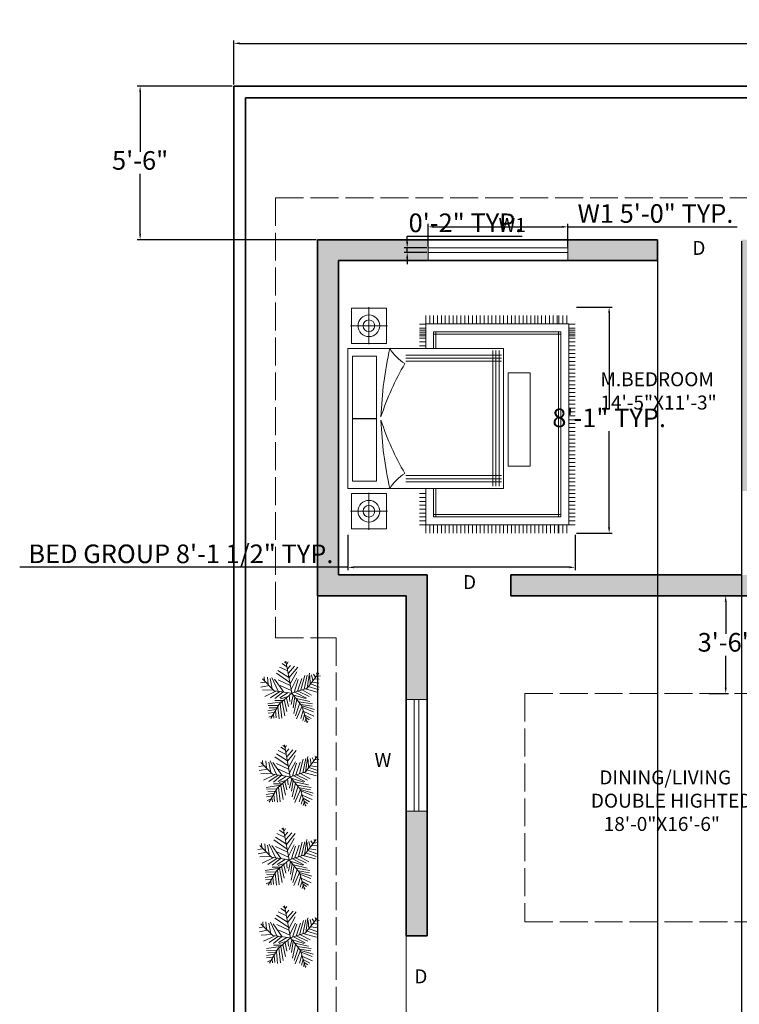
# Model space of a CAD drawing. Units: inches. Extents: x 1070 to 2371, y 645 to 1546.
# Tile 6 of 10: x 1070 to 1379, y 1014 to 1437. Entities that reach past the tile are written whole.
import ezdxf

# ---------------------------------------------------------------- set-up
doc = ezdxf.new("R2010")
doc.units = ezdxf.units.IN
doc.linetypes.add('ACAD_ISO02W100', pattern=[15, 12, -3])
for name, color, linetype, lineweight in [('A-ANNO-DIMS', 2, 'Continuous', 18), ('A-ANNO-TEXT', 7, 'Continuous', 18), ('A-AREA-IDEN', 7, 'Continuous', 18), ('A-DOOR', 4, 'Continuous', 18), ('A-FLOR-OVHD', 8, 'ACAD_ISO02W100', 13), ('A-FURN', 8, 'Continuous', 18), ('A-GLAZ', 4, 'Continuous', 18), ('A-ROOF-OVHD', 8, 'ACAD_ISO02W100', 13), ('A-WALL', 7, 'Continuous', 35), ('C-PROP', 7, 'Continuous', 35), ('L-PLNT-TREE', 94, 'Continuous', 13)]:
    doc.layers.add(name, color=color, linetype=linetype, lineweight=lineweight)
doc.layers.add('A-WALL-PATT', color=162, linetype='Continuous', lineweight=13, true_color=0x044ac3)
doc.styles.get("Standard").update_dxf_attribs({"font": 'arial.ttf'})
doc.dimstyles.new('ISO-25', dxfattribs={"dimtxt": 8, "dimasz": 2.5, "dimexe": 1.25, "dimexo": 0.625, "dimtad": 1, "dimtih": 1, "dimtoh": 1, "dimdec": 1, "dimlunit": 3, "dimtxsty": 'Standard', "dimcen": 2.5, "dimadec": 0, "dimazin": 0, "dimtfac": 1, "dimtdec": 1, "dimtmove": 0, "dimatfit": 3, "dimfxl": 1, "dimarcsym": 0})

# ---------------------------------------------------------------- blocks, each defined once
blk = doc.blocks.new('*U5')
for p, q in [((-8.737, 47.138), (-17.069, 52.711)), ((-10.186, 53.64), (-13.084, 55.962)), ((0, 0), (-10.5, 57)), ((-9.099, 51.782), (-6.563, 55.962)), ((-3.665, 19.273), (-27.574, 35.527)), ((-5.114, 28.097), (-24.676, 40.636)), ((-7.288, 39.707), (-21.778, 46.673)), ((-7.65, 43.423), (-2.578, 49.46)), ((-5.839, 35.992), (4.667, 48.067)), ((-5.114, 27.632), (10.463, 46.673)), ((-2.941, 16.486), (8.652, 37.85)), ((27, 9), (48, 36)), ((27.127, 9.056), (31.112, 35.992)), ((44.153, 36.456), (45.239, 32.741)), ((-47.498, 19.737), (-55.83, 18.344)), ((-31.5, 4.5), (-52.5, 25.5)), ((-48.585, 21.131), (-49.309, 29.026)), ((-43.513, 28.561), (-42.427, 15.558)), ((-38.442, 26.239), (-34.819, 7.663)), ((-35.544, 28.097), (-24.314, 3.947)), ((-14.533, 2.09), (-30.834, 25.31)), ((-24.314, 23.917), (-2.941, 13.7)), ((-1.129, 6.734), (9.014, 26.704)), ((3.942, 1.625), (11.187, 24.381)), ((10.101, 3.483), (17.708, 26.239)), ((16.259, 5.805), (23.142, 31.348)), ((22.055, 7.198), (27.489, 32.277)), ((31.836, 30.883), (32.561, 16.486)), ((35.096, 32.741), (37.27, 22.524)), ((36.183, 19.737), (48.137, 17.88)), ((38.719, 34.134), (41.979, 28.561)), ((40.53, 25.775), (48.862, 24.846)), ((43.791, 29.954), (51.036, 30.883)), ((-40.615, 13.7), (-55.105, 10.913)), ((-33.37, 6.269), (-52.207, 5.34)), ((-28.299, 3.483), (-47.86, -5.805)), ((-21.416, 3.018), (-38.079, -8.128)), ((0, 0), (-31.5, 4.5)), ((-15.982, 2.09), (-30.11, -9.521)), ((0, 0), (-22.5, -19.5)), ((-6.563, 1.161), (-21.416, -8.128)), ((-20.691, 13.7), (-1.129, 4.876)), ((0, 0), (27, 9)), ((0, 0), (18, -22.5)), ((6.478, 1.625), (26.04, -8.592)), ((11.187, 3.483), (30.749, -5.805)), ((18.07, 5.805), (35.096, -3.483)), ((24.229, 7.663), (46.688, 1.625)), ((29.662, 12.307), (48.137, 6.269)), ((33.285, 16.486), (48.862, 10.913)), ((-17.431, -15.094), (-42.789, -18.809)), ((-15.257, -12.772), (-30.11, -12.772)), ((-6.563, -5.805), (-19.967, -9.985)), ((-17.069, -15.094), (-12.721, -40.172)), ((-13.446, -11.378), (-8.737, -32.741)), ((-9.461, -8.592), (-6.201, -23.453)), ((-4.752, -3.483), (-3.665, -14.629)), ((2.493, -3.019), (-1.491, -20.202)), ((1.769, -2.555), (24.229, -9.521)), ((5.029, -6.27), (2.131, -25.775)), ((9.014, -11.378), (3.58, -35.992)), ((14.085, -16.951), (6.478, -40.172)), ((7.565, -9.056), (32.198, -14.629)), ((12.274, -15.094), (36.907, -18.809)), ((-28.299, -29.026), (-42.789, -31.348)), ((-24.314, -21.596), (-42.427, -22.06)), ((-30.834, -34.135), (-42.427, -35.528)), ((-26.849, -26.24), (-40.253, -25.775)), ((-22.5, -19.5), (-37.5, -45)), ((-29.023, -30.884), (-27.936, -43.887)), ((-25.038, -23.918), (-22.865, -45.281)), ((-20.691, -18.345), (-17.793, -44.352)), ((18.07, -22.524), (8.289, -45.745)), ((20.244, -30.419), (15.897, -44.816)), ((16.259, -19.738), (36.183, -22.989)), ((18, -22.5), (27, -52.5)), ((18.433, -22.524), (40.53, -29.026)), ((19.157, -25.311), (38.719, -33.206)), ((21.331, -32.741), (39.081, -40.636)), ((-34.457, -39.708), (-40.978, -42.494)), ((-32.646, -36.921), (-31.921, -44.352)), ((22.78, -37.85), (19.519, -48.532)), ((22.78, -38.314), (34.372, -44.816)), ((24.591, -45.745), (23.142, -50.854)), ((24.591, -43.423), (30.749, -47.603)), ((26.764, -49.925), (28.213, -50.854))]:
    blk.add_line(p, q)
blk = doc.blocks.new('A$C462B680F')
for p, q in [((2.33, 2.918, -0.291), (0.53, 2.918, -0.291)), ((0.53, 2.918, -0.291), (0.53, 0.918, -0.291)), ((2.33, 0.918, -0.291), (2.33, 2.918, -0.291)), ((0.011, 2.874, -0.291), (0.465, 2.874, -0.291)), ((0.011, 2.424, -0.291), (0.011, 2.874, -0.291)), ((0.238, 2.649, -0.561), (0.238, 2.887, -0.561)), ((0.465, 2.874, -0.291), (0.465, 2.424, -0.291)), ((1.434, 2.861, -0.291), (0.627, 2.861, -0.291)), ((0.627, 2.861, -0.291), (0.627, 2.55, -0.291)), ((1.43, 2.861, -0.291), (1.43, 2.55, -0.291)), ((2.237, 2.861, -0.291), (1.43, 2.861, -0.291)), ((1.434, 2.55, -0.291), (1.434, 2.861, -0.291)), ((2.237, 2.55, -0.291), (2.237, 2.861, -0.291)), ((2.849, 2.874, -0.291), (2.395, 2.874, -0.291)), ((2.395, 2.874, -0.291), (2.395, 2.424, -0.291)), ((2.622, 2.649, -0.561), (2.622, 2.887, -0.561)), ((2.849, 2.424, -0.291), (2.849, 2.874, -0.291)), ((0.238, 2.649, -0.561), (0, 2.649, -0.561)), ((0.238, 2.649, -0.561), (0.238, 2.411, -0.561)), ((0.238, 2.649, -0.561), (0.476, 2.649, -0.561)), ((0.627, 2.55, -0.291), (1.434, 2.55, -0.291)), ((1.43, 2.55, -0.291), (2.237, 2.55, -0.291)), ((2.622, 2.649, -0.561), (2.384, 2.649, -0.561)), ((2.622, 2.649, -0.561), (2.622, 2.411, -0.561)), ((2.622, 2.649, -0.561), (2.861, 2.649, -0.561)), ((0.465, 2.424, -0.291), (0.011, 2.424, -0.291)), ((2.395, 2.424, -0.291), (2.849, 2.424, -0.291)), ((0.615, 2.176, -0.291), (0.615, 0.947, -0.291)), ((0.655, 2.176, -0.291), (0.655, 0.947, -0.291)), ((0.695, 2.176, -0.291), (0.695, 0.947, -0.291)), ((2.165, 2.176, -0.291), (2.165, 0.947, -0.291)), ((2.205, 2.176, -0.291), (2.205, 0.947, -0.291)), ((2.245, 2.176, -0.291), (2.245, 0.947, -0.291)), ((0.215, 1.918, -0.291), (0.105, 1.918, -0.291)), ((0.215, 1.918, -0.291), (0.215, 0.082, -0.291)), ((0.53, 1.918, -0.291), (0.215, 1.918, -0.291)), ((0.219, 1.918, -0.291), (0.219, 2, -0.291)), ((0.269, 1.918, -0.291), (0.269, 2, -0.291)), ((0.296, 1.918, -0.291), (0.296, 2, -0.291)), ((0.319, 1.918, -0.291), (0.319, 2, -0.291)), ((0.346, 1.918, -0.291), (0.346, 2, -0.291)), ((0.369, 1.918, -0.291), (0.369, 2, -0.291)), ((0.396, 1.918, -0.291), (0.396, 2, -0.291)), ((0.446, 1.918, -0.291), (0.446, 2, -0.291)), ((0.496, 1.918, -0.291), (0.496, 2, -0.291)), ((2.33, 1.918, -0.291), (2.796, 1.918, -0.291)), ((2.396, 1.918, -0.291), (2.396, 2, -0.291)), ((2.446, 1.918, -0.291), (2.446, 2, -0.291)), ((2.496, 1.918, -0.291), (2.496, 2, -0.291)), ((2.546, 1.918, -0.291), (2.546, 2, -0.291)), ((2.596, 1.918, -0.291), (2.596, 2, -0.291)), ((2.646, 1.918, -0.291), (2.646, 2, -0.291)), ((2.696, 1.918, -0.291), (2.696, 2, -0.291)), ((2.746, 1.918, -0.291), (2.746, 2, -0.291)), ((2.796, 1.918, -0.291), (2.796, 2, -0.291)), ((2.796, 1.918, -0.291), (2.796, 0.082, -0.291)), ((2.796, 1.918, -0.291), (2.906, 1.918, -0.291)), ((0.215, 1.868, -0.291), (0.105, 1.868, -0.291)), ((0.215, 1.818, -0.291), (0.105, 1.818, -0.291)), ((0.315, 1.818, -0.291), (0.315, 0.182, -0.291)), ((0.53, 1.818, -0.291), (0.315, 1.818, -0.291)), ((0.53, 1.788, -0.291), (0.315, 1.788, -0.291)), ((0.345, 1.818, -0.291), (0.345, 0.182, -0.291)), ((2.33, 1.818, -0.291), (2.696, 1.818, -0.291)), ((2.33, 1.788, -0.291), (2.696, 1.788, -0.291)), ((2.666, 1.818, -0.291), (2.666, 0.182, -0.291)), ((2.696, 1.818, -0.291), (2.696, 0.182, -0.291)), ((2.796, 1.868, -0.291), (2.906, 1.868, -0.291)), ((2.796, 1.818, -0.291), (2.906, 1.818, -0.291)), ((0.215, 1.768, -0.291), (0.105, 1.768, -0.291)), ((0.215, 1.718, -0.291), (0.105, 1.718, -0.291)), ((0.215, 1.668, -0.291), (0.105, 1.668, -0.291)), ((2.796, 1.768, -0.291), (2.906, 1.768, -0.291)), ((2.796, 1.718, -0.291), (2.906, 1.718, -0.291)), ((2.796, 1.668, -0.291), (2.906, 1.668, -0.291)), ((0.215, 1.618, -0.291), (0.105, 1.618, -0.291)), ((0.215, 1.568, -0.291), (0.105, 1.568, -0.291)), ((2.796, 1.618, -0.291), (2.906, 1.618, -0.291)), ((2.796, 1.568, -0.291), (2.906, 1.568, -0.291)), ((0.215, 1.518, -0.291), (0.105, 1.518, -0.291)), ((0.215, 1.468, -0.291), (0.105, 1.468, -0.291)), ((0.215, 1.418, -0.291), (0.105, 1.418, -0.291)), ((2.796, 1.518, -0.291), (2.906, 1.518, -0.291)), ((2.796, 1.468, -0.291), (2.906, 1.468, -0.291)), ((2.796, 1.418, -0.291), (2.906, 1.418, -0.291)), ((0.215, 1.368, -0.291), (0.105, 1.368, -0.291)), ((0.215, 1.318, -0.291), (0.105, 1.318, -0.291)), ((0.215, 1.268, -0.291), (0.105, 1.268, -0.291)), ((2.796, 1.368, -0.291), (2.906, 1.368, -0.291)), ((2.796, 1.318, -0.291), (2.906, 1.318, -0.291)), ((2.796, 1.268, -0.291), (2.906, 1.268, -0.291)), ((0.215, 1.218, -0.291), (0.105, 1.218, -0.291)), ((0.215, 1.168, -0.291), (0.105, 1.168, -0.291)), ((2.796, 1.218, -0.291), (2.906, 1.218, -0.291)), ((2.796, 1.168, -0.291), (2.906, 1.168, -0.291)), ((0.215, 1.118, -0.291), (0.105, 1.118, -0.291)), ((0.215, 1.068, -0.291), (0.105, 1.068, -0.291)), ((0.215, 1.018, -0.291), (0.105, 1.018, -0.291)), ((0.558, 1.057, -0.291), (2.299, 1.057, -0.291)), ((0.558, 1.017, -0.291), (2.299, 1.017, -0.291)), ((2.796, 1.118, -0.291), (2.906, 1.118, -0.291)), ((2.796, 1.068, -0.291), (2.906, 1.068, -0.291)), ((2.796, 1.018, -0.291), (2.906, 1.018, -0.291)), ((0.215, 0.968, -0.291), (0.105, 0.968, -0.291)), ((0.215, 0.918, -0.291), (0.105, 0.918, -0.291)), ((0.53, 0.918, -0.291), (2.33, 0.918, -0.291)), ((0.558, 0.977, -0.291), (2.299, 0.977, -0.291)), ((2.796, 0.968, -0.291), (2.906, 0.968, -0.291)), ((2.796, 0.918, -0.291), (2.906, 0.918, -0.291)), ((0.215, 0.868, -0.291), (0.105, 0.868, -0.291)), ((0.215, 0.818, -0.291), (0.105, 0.818, -0.291)), ((0.215, 0.768, -0.291), (0.105, 0.768, -0.291)), ((0.844, 0.859, -0.291), (0.844, 0.579, -0.291)), ((2.044, 0.859, -0.291), (0.844, 0.859, -0.291)), ((2.044, 0.579, -0.291), (2.044, 0.859, -0.291)), ((2.796, 0.868, -0.291), (2.906, 0.868, -0.291)), ((2.796, 0.818, -0.291), (2.906, 0.818, -0.291)), ((2.796, 0.768, -0.291), (2.906, 0.768, -0.291)), ((0.215, 0.718, -0.291), (0.105, 0.718, -0.291)), ((0.215, 0.668, -0.291), (0.105, 0.668, -0.291)), ((2.796, 0.718, -0.291), (2.906, 0.718, -0.291)), ((2.796, 0.668, -0.291), (2.906, 0.668, -0.291)), ((0.215, 0.618, -0.291), (0.105, 0.618, -0.291)), ((0.215, 0.568, -0.291), (0.105, 0.568, -0.291)), ((0.215, 0.518, -0.291), (0.105, 0.518, -0.291)), ((0.844, 0.579, -0.291), (2.044, 0.579, -0.291)), ((2.796, 0.618, -0.291), (2.906, 0.618, -0.291)), ((2.796, 0.568, -0.291), (2.906, 0.568, -0.291)), ((2.796, 0.518, -0.291), (2.906, 0.518, -0.291)), ((2.796, 0.516, -0.291), (2.906, 0.516, -0.291)), ((0.215, 0.48, -0.291), (0.105, 0.48, -0.291)), ((0.215, 0.43, -0.291), (0.105, 0.43, -0.291)), ((0.215, 0.38, -0.291), (0.105, 0.38, -0.291)), ((2.796, 0.466, -0.291), (2.906, 0.466, -0.291)), ((2.796, 0.416, -0.291), (2.906, 0.416, -0.291)), ((0.215, 0.33, -0.291), (0.105, 0.33, -0.291)), ((0.215, 0.28, -0.291), (0.105, 0.28, -0.291)), ((2.796, 0.366, -0.291), (2.906, 0.366, -0.291)), ((2.796, 0.316, -0.291), (2.906, 0.316, -0.291)), ((2.796, 0.266, -0.291), (2.906, 0.266, -0.291)), ((0.215, 0.23, -0.291), (0.105, 0.23, -0.291)), ((0.215, 0.207, -0.291), (0.105, 0.207, -0.291)), ((0.215, 0.207, -0.291), (0.105, 0.207, -0.291)), ((0.215, 0.157, -0.291), (0.105, 0.157, -0.291)), ((2.696, 0.212, -0.291), (0.315, 0.212, -0.291)), ((2.696, 0.182, -0.291), (0.315, 0.182, -0.291)), ((2.796, 0.216, -0.291), (2.906, 0.216, -0.291)), ((2.796, 0.207, -0.291), (2.906, 0.207, -0.291)), ((2.796, 0.207, -0.291), (2.906, 0.207, -0.291)), ((2.796, 0.157, -0.291), (2.906, 0.157, -0.291)), ((0.215, 0.107, -0.291), (0.105, 0.107, -0.291)), ((2.796, 0.082, -0.291), (0.215, 0.082, -0.291)), ((0.219, 0.082, -0.291), (0.219, 0, -0.291)), ((0.269, 0.082, -0.291), (0.269, 0, -0.291)), ((0.296, 0.082, -0.291), (0.296, 0, -0.291)), ((0.319, 0.082, -0.291), (0.319, 0, -0.291)), ((0.346, 0.082, -0.291), (0.346, 0, -0.291)), ((0.369, 0.082, -0.291), (0.369, 0, -0.291)), ((0.396, 0.082, -0.291), (0.396, 0, -0.291)), ((0.446, 0.082, -0.291), (0.446, 0, -0.291)), ((0.496, 0.082, -0.291), (0.496, 0, -0.291)), ((0.546, 0.082, -0.291), (0.546, 0, -0.291)), ((0.596, 0.082, -0.291), (0.596, 0, -0.291)), ((0.646, 0.082, -0.291), (0.646, 0, -0.291)), ((0.696, 0.082, -0.291), (0.696, 0, -0.291)), ((0.746, 0.082, -0.291), (0.746, 0, -0.291)), ((0.796, 0.082, -0.291), (0.796, 0, -0.291)), ((0.846, 0.082, -0.291), (0.846, 0, -0.291)), ((0.896, 0.082, -0.291), (0.896, 0, -0.291)), ((0.946, 0.082, -0.291), (0.946, 0, -0.291)), ((0.996, 0.082, -0.291), (0.996, 0, -0.291)), ((1.046, 0.082, -0.291), (1.046, 0, -0.291)), ((1.096, 0.082, -0.291), (1.096, 0, -0.291)), ((1.146, 0.082, -0.291), (1.146, 0, -0.291)), ((1.196, 0.082, -0.291), (1.196, 0, -0.291)), ((1.246, 0.082, -0.291), (1.246, 0, -0.291)), ((1.296, 0.082, -0.291), (1.296, 0, -0.291)), ((1.346, 0.082, -0.291), (1.346, 0, -0.291)), ((1.346, 0.082, -0.291), (1.346, 0, -0.291)), ((1.396, 0.082, -0.291), (1.396, 0, -0.291)), ((1.396, 0.082, -0.291), (1.396, 0, -0.291)), ((1.446, 0.082, -0.291), (1.446, 0, -0.291)), ((1.446, 0.082, -0.291), (1.446, 0, -0.291)), ((1.496, 0.082, -0.291), (1.496, 0, -0.291)), ((1.496, 0.082, -0.291), (1.496, 0, -0.291)), ((1.546, 0.082, -0.291), (1.546, 0, -0.291)), ((1.596, 0.082, -0.291), (1.596, 0, -0.291)), ((1.646, 0.082, -0.291), (1.646, 0, -0.291)), ((1.696, 0.082, -0.291), (1.696, 0, -0.291)), ((1.746, 0.082, -0.291), (1.746, 0, -0.291)), ((1.796, 0.082, -0.291), (1.796, 0, -0.291)), ((1.846, 0.082, -0.291), (1.846, 0, -0.291)), ((1.846, 0.082, -0.291), (1.846, 0, -0.291)), ((1.896, 0.082, -0.291), (1.896, 0, -0.291)), ((1.946, 0.082, -0.291), (1.946, 0, -0.291)), ((1.996, 0.082, -0.291), (1.996, 0, -0.291)), ((2.046, 0.082, -0.291), (2.046, 0, -0.291)), ((2.096, 0.082, -0.291), (2.096, 0, -0.291)), ((2.146, 0.082, -0.291), (2.146, 0, -0.291)), ((2.196, 0.082, -0.291), (2.196, 0, -0.291)), ((2.246, 0.082, -0.291), (2.246, 0, -0.291)), ((2.296, 0.082, -0.291), (2.296, 0, -0.291)), ((2.346, 0.082, -0.291), (2.346, 0, -0.291)), ((2.396, 0.082, -0.291), (2.396, 0, -0.291)), ((2.446, 0.082, -0.291), (2.446, 0, -0.291)), ((2.496, 0.082, -0.291), (2.496, 0, -0.291)), ((2.546, 0.082, -0.291), (2.546, 0, -0.291)), ((2.596, 0.082, -0.291), (2.596, 0, -0.291)), ((2.646, 0.082, -0.291), (2.646, 0, -0.291)), ((2.696, 0.082, -0.291), (2.696, 0, -0.291)), ((2.746, 0.082, -0.291), (2.746, 0, -0.291)), ((2.796, 0.107, -0.291), (2.906, 0.107, -0.291)), ((2.796, 0.082, -0.291), (2.796, 0, -0.291))]:
    blk.add_line(p, q)
for centre, radius in [((0.238, 2.649, -0.561), 0.139), ((2.622, 2.649, -0.561), 0.139), ((0.238, 2.649, -0.561), 0.075), ((2.622, 2.649, -0.561), 0.075)]:
    blk.add_circle(centre, radius)
for centre, radius, start, end in [((1.618, -2.572, -0.291), 5.071, 92.3872, 102.3913), ((2.601, -1.074, -0.291), 3.763, 108.5127, 119.9306), ((1.243, -2.572, -0.291), 5.071, 77.6087, 87.6128), ((0.259, -1.074, -0.291), 3.763, 60.0694, 71.4873), ((0.231, 1.886, -0.291), 0.578, 31.4118, 58.8491), ((2.63, 1.886, -0.291), 0.578, 121.1509, 148.5882)]:
    blk.add_arc(centre, radius, start, end)
blk = doc.blocks.new('*D11')
at = {"layer": 'A-ANNO-DIMS', "color": 0, "lineweight": -2, "transparency": 16777216}
for p, q in [((1162.11, 1409.4), (1162.11, 1428.36)), ((1164.61, 1427.11), (1639.61, 1427.11)), ((1642.11, 1409.4), (1642.11, 1428.36))]:
    blk.add_line(p, q, dxfattribs=at)
at = {"layer": 'A-ANNO-DIMS', "color": 0, "transparency": 16777216}
for points in [[(1164.61, 1427.53), (1164.61, 1426.7), (1162.11, 1427.11)], [(1639.61, 1427.53), (1639.61, 1426.7), (1642.11, 1427.11)]]:
    blk.add_solid(points, dxfattribs=at)
at = {"layer": 'Defpoints', "color": 0, "transparency": 16777216}
for p in [(1642.11, 1427.11), (1162.11, 1408.77), (1642.11, 1408.77)]:
    blk.add_point(p, dxfattribs=at)
at = {"layer": 'A-ANNO-DIMS', "color": 0, "transparency": 16777216, "insert": (1402.11, 1431.82), "char_height": 8, "attachment_point": 5}
blk.add_mtext("40'", dxfattribs=at)
blk = doc.blocks.new('*D13')
at = {"layer": 'A-ANNO-DIMS', "color": 0, "lineweight": -2, "transparency": 16777216}
for p, q in [((1366.14, 1189.77), (1374.63, 1189.77)), ((1373.38, 1187.27), (1373.38, 1173.48)), ((1373.38, 1150.27), (1373.38, 1164.06)), ((1366.14, 1147.77), (1374.63, 1147.77))]:
    blk.add_line(p, q, dxfattribs=at)
at = {"layer": 'A-ANNO-DIMS', "color": 0, "transparency": 16777216}
for points in [[(1372.97, 1187.27), (1373.8, 1187.27), (1373.38, 1189.77)], [(1372.97, 1150.27), (1373.8, 1150.27), (1373.38, 1147.77)]]:
    blk.add_solid(points, dxfattribs=at)
at = {"layer": 'Defpoints', "color": 0, "transparency": 16777216}
for p in [(1365.51, 1189.77), (1365.51, 1147.77), (1373.38, 1147.77)]:
    blk.add_point(p, dxfattribs=at)
at = {"layer": 'A-ANNO-DIMS', "color": 0, "transparency": 16777216, "insert": (1373.38, 1168.77), "char_height": 8, "attachment_point": 5}
blk.add_mtext('3\'-6"', dxfattribs=at)
blk = doc.blocks.new('GLAZ-48IN')
for p, q in [((0, 48), (0, 0)), ((2, 48), (2, 0))]:
    blk.add_line(p, q)
blk = doc.blocks.new('GLAZ-60IN')
for p, q in [((60, 2), (0, 2)), ((60, 0), (0, 0))]:
    blk.add_line(p, q)
blk = doc.blocks.new('*D27')
at = {"layer": 'A-ANNO-DIMS', "color": 0, "lineweight": -2, "transparency": 16777216}
for p, q in [((1211.17, 1216.02), (1211.17, 1200.77)), ((1308.69, 1216.02), (1308.69, 1200.77)), ((1211.17, 1202.02), (1070.2, 1202.02)), ((1306.19, 1202.02), (1213.67, 1202.02))]:
    blk.add_line(p, q, dxfattribs=at)
at = {"layer": 'A-ANNO-DIMS', "color": 0, "transparency": 16777216}
for points in [[(1213.67, 1202.44), (1213.67, 1201.6), (1211.17, 1202.02)], [(1306.19, 1202.44), (1306.19, 1201.6), (1308.69, 1202.02)]]:
    blk.add_solid(points, dxfattribs=at)
at = {"layer": 'Defpoints', "color": 0, "transparency": 16777216}
for p in [(1211.17, 1216.65), (1308.69, 1216.65), (1211.17, 1202.02)]:
    blk.add_point(p, dxfattribs=at)
at = {"layer": 'A-ANNO-DIMS', "color": 0, "transparency": 16777216, "insert": (1139.43, 1206.78), "char_height": 8, "attachment_point": 5}
blk.add_mtext('BED GROUP 8\'-1 1/2" TYP.', dxfattribs=at)
blk = doc.blocks.new('*D28')
at = {"layer": 'A-ANNO-DIMS', "color": 0, "lineweight": -2, "transparency": 16777216}
for p, q in [((1309.32, 1313.75), (1324.57, 1313.75)), ((1323.32, 1311.25), (1323.32, 1269.91)), ((1323.32, 1219.15), (1323.32, 1260.49)), ((1309.32, 1216.65), (1324.57, 1216.65))]:
    blk.add_line(p, q, dxfattribs=at)
at = {"layer": 'A-ANNO-DIMS', "color": 0, "transparency": 16777216}
for points in [[(1322.9, 1311.25), (1323.74, 1311.25), (1323.32, 1313.75)], [(1322.9, 1219.15), (1323.74, 1219.15), (1323.32, 1216.65)]]:
    blk.add_solid(points, dxfattribs=at)
at = {"layer": 'Defpoints', "color": 0, "transparency": 16777216}
for p in [(1308.69, 1313.75), (1308.69, 1216.65), (1323.32, 1216.65)]:
    blk.add_point(p, dxfattribs=at)
at = {"layer": 'A-ANNO-DIMS', "color": 0, "transparency": 16777216, "insert": (1323.32, 1265.2), "char_height": 8, "attachment_point": 5}
blk.add_mtext('8\'-1" TYP.', dxfattribs=at)
blk = doc.blocks.new('*D41')
at = {"layer": 'A-ANNO-DIMS', "color": 0, "lineweight": -2, "transparency": 16777216}
for p, q in [((1245.61, 1339.9), (1245.61, 1349.52)), ((1305.61, 1339.9), (1305.61, 1349.52)), ((1248.11, 1348.27), (1303.11, 1348.27)), ((1305.61, 1348.27), (1378.32, 1348.27))]:
    blk.add_line(p, q, dxfattribs=at)
at = {"layer": 'A-ANNO-DIMS', "color": 0, "transparency": 16777216}
for points in [[(1248.11, 1348.69), (1248.11, 1347.86), (1245.61, 1348.27)], [(1303.11, 1348.69), (1303.11, 1347.86), (1305.61, 1348.27)]]:
    blk.add_solid(points, dxfattribs=at)
at = {"layer": 'Defpoints', "color": 0, "transparency": 16777216}
for p in [(1305.61, 1348.27), (1245.61, 1339.27), (1305.61, 1339.27)]:
    blk.add_point(p, dxfattribs=at)
at = {"layer": 'A-ANNO-DIMS', "color": 0, "transparency": 16777216, "insert": (1343.22, 1352.98), "char_height": 8, "attachment_point": 5}
blk.add_mtext('W1 5\'-0" TYP.', dxfattribs=at)
blk = doc.blocks.new('*D42')
at = {"layer": 'A-ANNO-DIMS', "color": 0, "lineweight": -2, "transparency": 16777216}
for p, q in [((1236.61, 1341.77), (1236.61, 1344.27)), ((1236.61, 1344.27), (1286, 1344.27)), ((1244.99, 1339.27), (1235.36, 1339.27)), ((1244.99, 1337.27), (1235.36, 1337.27)), ((1236.61, 1337.27), (1236.61, 1339.27)), ((1236.61, 1334.77), (1236.61, 1332.27))]:
    blk.add_line(p, q, dxfattribs=at)
at = {"layer": 'A-ANNO-DIMS', "color": 0, "transparency": 16777216}
for points in [[(1236.2, 1341.77), (1237.03, 1341.77), (1236.61, 1339.27)], [(1236.2, 1334.77), (1237.03, 1334.77), (1236.61, 1337.27)]]:
    blk.add_solid(points, dxfattribs=at)
at = {"layer": 'Defpoints', "color": 0, "transparency": 16777216}
for p in [(1236.61, 1339.27), (1245.61, 1339.27), (1245.61, 1337.27)]:
    blk.add_point(p, dxfattribs=at)
at = {"layer": 'A-ANNO-DIMS', "color": 0, "transparency": 16777216, "insert": (1261.62, 1348.98), "char_height": 8, "attachment_point": 5}
blk.add_mtext('0\'-2" TYP.', dxfattribs=at)
blk = doc.blocks.new('*D47')
at = {"layer": 'A-ANNO-DIMS', "color": 0, "lineweight": -2, "transparency": 16777216}
for p, q in [((1162.11, 1408.15), (1162.11, 647.32)), ((1198.11, 1342.15), (1198.11, 647.32)), ((1164.61, 648.57), (1195.61, 648.57))]:
    blk.add_line(p, q, dxfattribs=at)
at = {"layer": 'A-ANNO-DIMS', "color": 0, "transparency": 16777216}
for points in [[(1164.61, 648.99), (1164.61, 648.16), (1162.11, 648.57)], [(1195.61, 648.99), (1195.61, 648.16), (1198.11, 648.57)]]:
    blk.add_solid(points, dxfattribs=at)
at = {"layer": 'Defpoints', "color": 0, "transparency": 16777216}
for p in [(1162.11, 1408.77), (1198.11, 1342.77), (1198.11, 648.57)]:
    blk.add_point(p, dxfattribs=at)
at = {"layer": 'A-ANNO-DIMS', "color": 0, "transparency": 16777216, "insert": (1180.11, 653.28), "char_height": 8, "attachment_point": 5}
blk.add_mtext('3\'-0"', dxfattribs=at)
blk = doc.blocks.new('*D48')
at = {"layer": 'A-ANNO-DIMS', "color": 0, "lineweight": -2, "transparency": 16777216}
for p, q in [((1161.49, 1408.77), (1120.66, 1408.77)), ((1121.91, 1406.27), (1121.91, 1380.48)), ((1121.91, 1345.27), (1121.91, 1371.06)), ((1197.49, 1342.77), (1120.66, 1342.77))]:
    blk.add_line(p, q, dxfattribs=at)
at = {"layer": 'A-ANNO-DIMS', "color": 0, "transparency": 16777216}
for points in [[(1121.5, 1406.27), (1122.33, 1406.27), (1121.91, 1408.77)], [(1121.5, 1345.27), (1122.33, 1345.27), (1121.91, 1342.77)]]:
    blk.add_solid(points, dxfattribs=at)
at = {"layer": 'Defpoints', "color": 0, "transparency": 16777216}
for p in [(1162.11, 1408.77), (1121.91, 1342.77), (1198.11, 1342.77)]:
    blk.add_point(p, dxfattribs=at)
at = {"layer": 'A-ANNO-DIMS', "color": 0, "transparency": 16777216, "insert": (1121.91, 1375.77), "char_height": 8, "attachment_point": 5}
blk.add_mtext('5\'-6"', dxfattribs=at)
blk = doc.blocks.new('*D49')
at = {"layer": 'A-ANNO-DIMS', "color": 0, "lineweight": -2, "transparency": 16777216}
for p, q in [((1344.11, 1342.15), (1344.11, 647.32)), ((1380.11, 1342.15), (1380.11, 647.32)), ((1346.61, 648.57), (1377.61, 648.57))]:
    blk.add_line(p, q, dxfattribs=at)
at = {"layer": 'A-ANNO-DIMS', "color": 0, "transparency": 16777216}
for points in [[(1346.61, 648.99), (1346.61, 648.16), (1344.11, 648.57)], [(1377.61, 648.99), (1377.61, 648.16), (1380.11, 648.57)]]:
    blk.add_solid(points, dxfattribs=at)
at = {"layer": 'Defpoints', "color": 0, "transparency": 16777216}
for p in [(1344.11, 1342.77), (1380.11, 1342.77), (1380.11, 648.57)]:
    blk.add_point(p, dxfattribs=at)
at = {"layer": 'A-ANNO-DIMS', "color": 0, "transparency": 16777216, "insert": (1362.11, 653.28), "char_height": 8, "attachment_point": 5}
blk.add_mtext('3\'-0"', dxfattribs=at)

msp = doc.modelspace()

# ---------------------------------------------------------------- hatches: boundary and pattern name
at = {"layer": 'A-WALL-PATT'}
h = msp.add_hatch(color=256, dxfattribs=at)
h.dxf.hatch_style = 1
h.paths.add_polyline_path([(1245.11, 1097.27), (1236.11, 1097.27), (1236.11, 1043.77), (1245.11, 1043.77)])
h.paths.add_polyline_path([(1245.11, 1198.77), (1207.11, 1198.77), (1207.11, 1333.77), (1245.61, 1333.77), (1245.61, 1342.77), (1198.11, 1342.77), (1198.11, 1189.77), (1236.11, 1189.77), (1236.11, 1145.27), (1245.11, 1145.27)])
h.paths.add_polyline_path([(1344.11, 1342.77), (1305.61, 1342.77), (1305.61, 1333.77), (1344.11, 1333.77)], flags=0)
h.paths.add_polyline_path([(1413.11, 1342.77), (1380.11, 1342.77), (1380.11, 1234.77), (1389.11, 1234.77), (1389.11, 1333.77), (1413.11, 1333.77)], flags=17)
h.paths.add_polyline_path([(1470.11, 1342.77), (1437.11, 1342.77), (1437.11, 1333.77), (1461.11, 1333.77), (1461.11, 1262.77), (1419.11, 1262.77), (1419.11, 1257.77), (1461.11, 1257.77), (1461.11, 1198.77), (1380.11, 1198.77), (1281.11, 1198.77), (1281.11, 1189.77), (1470.11, 1189.77)])
h.paths.add_polyline_path([(1524.61, 1300.77), (1506.11, 1300.77), (1506.11, 1291.77), (1524.61, 1291.77)], flags=17)
h.paths.add_polyline_path([(1600.11, 1300.77), (1572.61, 1300.77), (1572.61, 1291.77), (1591.11, 1291.77), (1591.11, 1152.77), (1461.11, 1152.77), (1461.11, 1143.77), (1567.11, 1143.77), (1567.11, 1131.77), (1576.11, 1131.77), (1576.11, 1143.77), (1600.11, 1143.77)])
h.paths.add_polyline_path([(1600.11, 1071.77), (1576.11, 1071.77), (1576.11, 1083.77), (1567.11, 1083.77), (1567.11, 1071.77), (1461.11, 1071.77), (1461.11, 1043.77), (1466.11, 1043.77), (1466.11, 1066.77), (1508.11, 1066.77), (1508.11, 1037.77), (1513.11, 1037.77), (1513.11, 1062.77), (1591.11, 1062.77), (1591.11, 1047.27), (1600.11, 1047.27)])
h.paths.add_polyline_path([(1600.11, 1023.27), (1591.11, 1023.27), (1591.11, 1007.77), (1461.11, 1007.77), (1461.11, 1002.77), (1591.11, 1002.77), (1591.11, 813.77), (1550.11, 813.77), (1550.11, 804.77), (1600.11, 804.77)])
h.paths.add_polyline_path([(1502.11, 813.77), (1461.11, 813.77), (1461.11, 804.77), (1502.11, 804.77)], flags=0)
h.paths.add_polyline_path([(1419.11, 1007.77), (1395.11, 1007.77), (1395.11, 998.77), (1410.11, 998.77), (1410.11, 916.77), (1395.11, 916.77), (1395.11, 907.77), (1410.11, 907.77), (1410.11, 804.77), (1419.11, 804.77)])
h = msp.add_hatch(color=256, dxfattribs=at)
h.dxf.hatch_style = 1
h.paths.add_polyline_path([(1344.11, 1342.77), (1305.61, 1342.77), (1305.61, 1333.77), (1344.11, 1333.77)])

# ---------------------------------------------------------------- linework, layer by layer
at = {"layer": 'A-DOOR'}
msp.add_line((1236.11, 1043.77), (1236.11, 1007.77), dxfattribs=at)
at = {"layer": 'A-FLOR-OVHD'}
for p, q in [((1287.11, 1147.77), (1419.11, 1147.77)), ((1287.11, 1147.77), (1287.11, 1049.77)), ((1287.11, 1049.77), (1419.11, 1049.77))]:
    msp.add_line(p, q, dxfattribs=at)
at = {"layer": 'A-GLAZ'}
for p, q in [((1245.61, 1333.77), (1245.61, 1342.77)), ((1305.61, 1333.77), (1305.61, 1342.77)), ((1245.11, 1145.27), (1236.11, 1145.27)), ((1245.11, 1097.27), (1236.11, 1097.27))]:
    msp.add_line(p, q, dxfattribs=at)
at = {"layer": 'A-ROOF-OVHD'}
for p, q in [((1180.11, 1360.77), (1180.11, 1171.77)), ((1180.11, 1360.77), (1389.11, 1360.77)), ((1180.11, 1171.77), (1206.11, 1171.77)), ((1206.11, 1171.77), (1206.11, 1007.77))]:
    msp.add_line(p, q, dxfattribs=at)
at = {"layer": 'A-WALL'}
for p, q in [((1198.11, 1342.77), (1198.11, 1189.77)), ((1198.11, 1342.77), (1344.11, 1342.77)), ((1344.11, 1342.77), (1344.11, 1333.77)), ((1207.11, 1333.77), (1207.11, 1198.77)), ((1207.11, 1333.77), (1344.11, 1333.77)), ((1207.11, 1198.77), (1245.11, 1198.77)), ((1245.11, 1198.77), (1245.11, 1043.77)), ((1281.11, 1198.77), (1281.11, 1189.77)), ((1281.11, 1198.77), (1380.11, 1198.77)), ((1198.11, 1189.77), (1236.11, 1189.77)), ((1236.11, 1189.77), (1236.11, 1043.77)), ((1281.11, 1189.77), (1470.11, 1189.77)), ((1236.11, 1043.77), (1245.11, 1043.77))]:
    msp.add_line(p, q, dxfattribs=at)
at = {"layer": 'C-PROP'}
for p, q in [((1162.11, 1408.77), (1162.11, 688.77)), ((1162.11, 1408.77), (1642.11, 1408.77)), ((1167.11, 1403.77), (1167.11, 693.77)), ((1167.11, 1403.77), (1637.11, 1403.77))]:
    msp.add_line(p, q, dxfattribs=at)

# ---------------------------------------------------------------- block references
at = {"layer": 'A-FURN', "xscale": -33.42019788357461, "yscale": 33.42019788357461, "zscale": 33.42019788357461, "rotation": 90}
msp.add_blockref('A$C462B680F', (1308.69, 1313.75, 9.72), dxfattribs=at)
at = {"layer": 'A-GLAZ'}
msp.add_blockref('GLAZ-60IN', (1245.61, 1337.27), dxfattribs=at)
at = {"layer": 'A-GLAZ', "rotation": 180}
msp.add_blockref('GLAZ-48IN', (1241.61, 1145.27), dxfattribs=at)
at = {"layer": 'L-PLNT-TREE', "xscale": 0.2412959654679437, "yscale": 0.2412959654679437, "zscale": 0.2412959654679437}
for p in [(1187.07, 1147.92), (1186.4, 1112.04), (1185.94, 1076.35), (1186.46, 1042.78)]:
    msp.add_blockref('*U5', p, dxfattribs=at)

# ---------------------------------------------------------------- texts
at = {"layer": 'A-ANNO-TEXT', "char_height": 6, "attachment_point": 1}
for s, insert in [('W1', (1275.84, 1352.09)), ('D', (1359.05, 1342.22)), ('D', (1260.56, 1198.66)), ('W', (1222.59, 1122.23)), ('D', (1239.65, 1029.29))]:
    msp.add_mtext_dynamic_manual_height_columns(s, width=20.5094, gutter_width=12.5, heights=[0], dxfattribs=dict(at, insert=insert))
at = {"layer": 'A-AREA-IDEN', "char_height": 6, "attachment_point": 1}
for s, width, insert in [('M.BEDROOM\\P14\'-5"X11\'-3"', 52.767, (1319.56, 1285.81)), ('  DINING/LIVING\\PDOUBLE HIGHTED\\P   18\'-0"X16\'-6"', 97.1991, (1315.46, 1114.77))]:
    msp.add_mtext_dynamic_manual_height_columns(s, width=width, gutter_width=12.5, heights=[0], dxfattribs=dict(at, insert=insert))

# ---------------------------------------------------------------- dimensions: what is measured, and where the dimension line sits
at = {"layer": 'A-ANNO-DIMS'}
for base, p1, p2, override, picture, middle in [((1642.11, 1427.11), (1162.11, 1408.77), (1642.11, 1408.77), {"dimclrd": 0, "dimclre": 0, "dimclrt": 0}, '*D11', (1402.11, 1431.82)), ((1198.11, 648.57), (1162.11, 1408.77), (1198.11, 1342.77), {"dimdec": 1, "dimlfac": 1, "dimrnd": 0, "dimzin": 1, "dimdsep": 46, "dimlunit": 4, "dimfrac": 2}, '*D47', (1180.11, 653.28)), ((1380.11, 648.57), (1344.11, 1342.77), (1380.11, 1342.77), {"dimdec": 1, "dimlfac": 1, "dimrnd": 0, "dimzin": 1, "dimdsep": 46, "dimlunit": 4, "dimfrac": 2}, '*D49', (1362.11, 653.28))]:
    dim = msp.add_linear_dim(base=base, p1=p1, p2=p2, dimstyle='ISO-25', override=override, dxfattribs=at)
    dim.commit()
    dim.dimension.update_dxf_attribs({"geometry": picture, "text_midpoint": middle})
for base, p1, p2, override, picture, middle in [((1121.91, 1342.77), (1162.11, 1408.77), (1198.11, 1342.77), {"dimdec": 1, "dimlfac": 1, "dimrnd": 0, "dimzin": 1, "dimdsep": 46, "dimlunit": 4, "dimfrac": 2}, '*D48', (1121.91, 1375.77)), ((1373.38, 1147.77), (1365.51, 1189.77), (1365.51, 1147.77), {"dimclrd": 0, "dimclre": 0, "dimclrt": 0}, '*D13', (1373.38, 1168.77))]:
    dim = msp.add_linear_dim(base=base, p1=p1, p2=p2, angle=90, dimstyle='ISO-25', override=override, dxfattribs=at)
    dim.commit()
    dim.dimension.update_dxf_attribs({"geometry": picture, "text_midpoint": middle})
dim = msp.add_linear_dim(base=(1305.61, 1348.27), p1=(1245.61, 1339.27), p2=(1305.61, 1339.27), text='W1 <> TYP.', dimstyle='ISO-25', override={"dimdec": 1, "dimlfac": 1, "dimrnd": 0, "dimzin": 1, "dimdsep": 46, "dimlunit": 4, "dimfrac": 2}, dxfattribs=at)
dim.commit()
dim.dimension.update_dxf_attribs({"geometry": '*D41', "text_midpoint": (1343.22, 1352.98)})
for base, p1, p2, angle, text, picture, middle in [((1236.61, 1339.27), (1245.61, 1337.27), (1245.61, 1339.27), 90, '<> TYP.', '*D42', (1261.62, 1348.98)), ((1323.32, 1216.65), (1308.69, 1313.75), (1308.69, 1216.65), 270, '<> TYP.', '*D28', (1323.32, 1265.2)), ((1211.17, 1202.02), (1308.69, 1216.65), (1211.17, 1216.65), 180, 'BED GROUP <> TYP.', '*D27', (1139.43, 1206.78))]:
    dim = msp.add_linear_dim(base=base, p1=p1, p2=p2, angle=angle, text=text, dimstyle='ISO-25', override={"dimdec": 1, "dimlfac": 1, "dimrnd": 0, "dimzin": 1, "dimdsep": 46, "dimlunit": 4, "dimfrac": 2}, dxfattribs=at)
    dim.commit()
    dim.dimension.update_dxf_attribs({"geometry": picture, "text_midpoint": middle})

doc.saveas('drawing.dxf')
